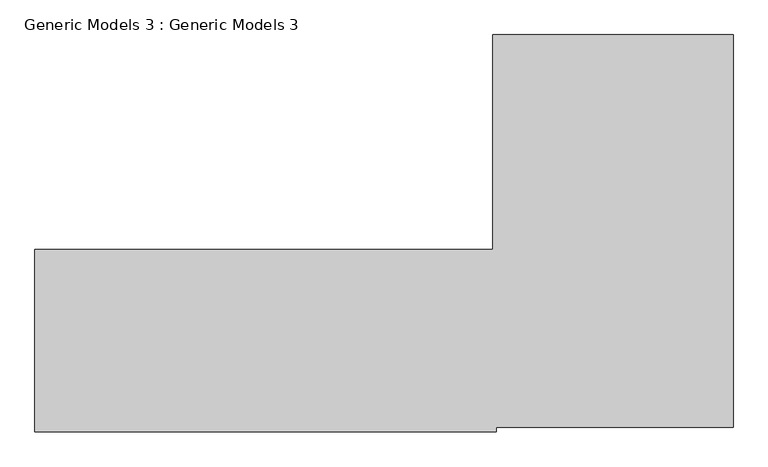
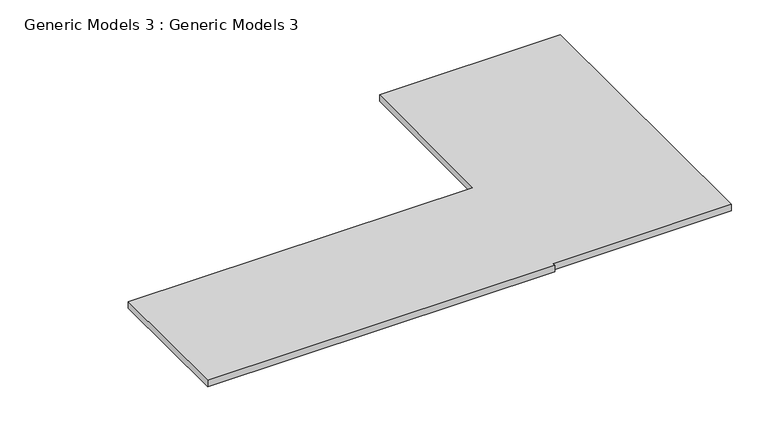
"""IFC4 building model written with IfcOpenShell, lengths in millimetres: proxy geometry, Generic Models 3 : Generic Models 3."""

from ifc_helpers import new_model, si_unit, origin, origin_with_axes, place, context, project, spatial, polyline, outline, extrude, source, transform, mapped, element, save


def generic_models_3_generic_models_3_d497b559(model_context):
    return source(origin(), model_context, "Body", "SweptSolid", [
        extrude(outline(polyline([(-20328.4535712, -4591.8496381), (-12683.0535712, -4591.8496381), (-12683.0535712, -1006.9606438), (-8669.8535712, -1006.9606438), (-8669.8535712, -7563.6496381), (-12626.4183666, -7563.6496381), (-12626.4183666, -7639.8496381), (-20328.4535712, -7639.8496381), (-20328.4535712, -4591.8496381)])), origin_with_axes(), (0.0, 0.0, 1.0), 152.4),
    ])


if __name__ == "__main__":
    model = new_model("IFC4")
    model_context = context("Model", 3, world=origin())
    ifc_project = project(units=[si_unit("LENGTHUNIT", "METRE", prefix="MILLI")], contexts=[model_context])
    site = spatial("IfcSite", under=ifc_project)
    building = spatial("IfcBuilding", under=site)
    placement = place(None, origin())
    generic_models_3_generic_models_3_shape = generic_models_3_generic_models_3_d497b559(model_context)
    element("IfcBuildingElementProxy", 1, Name="Generic Models 3 : Generic Models 3", ObjectType="Generic Models 3 : Generic Models 3", at=placement, inside=building, context=model_context, shape_type="MappedRepresentation", body=[
        mapped(generic_models_3_generic_models_3_shape, transform((0.0, 0.0, 0.0), x_axis=(1.0, 0.0, 0.0), y_axis=(0.0, 1.0, 0.0), z_axis=(0.0, 0.0, 1.0))),
    ])
    save(model, "model.ifc")

# Revit data of these elements
# Element 1 (IfcBuildingElementProxy, "Generic Models 3 : Generic Models 3")
#   Materials on its faces: "Acoustic Ceiling Tile 24 x 24"
# Materials
#   "Acoustic Ceiling Tile 24 x 24": class "Generic", colour RGB 232 232 232, transparency 0, Description = "Acoustic Ceiling Tile 24 x 24", Cost = 0
